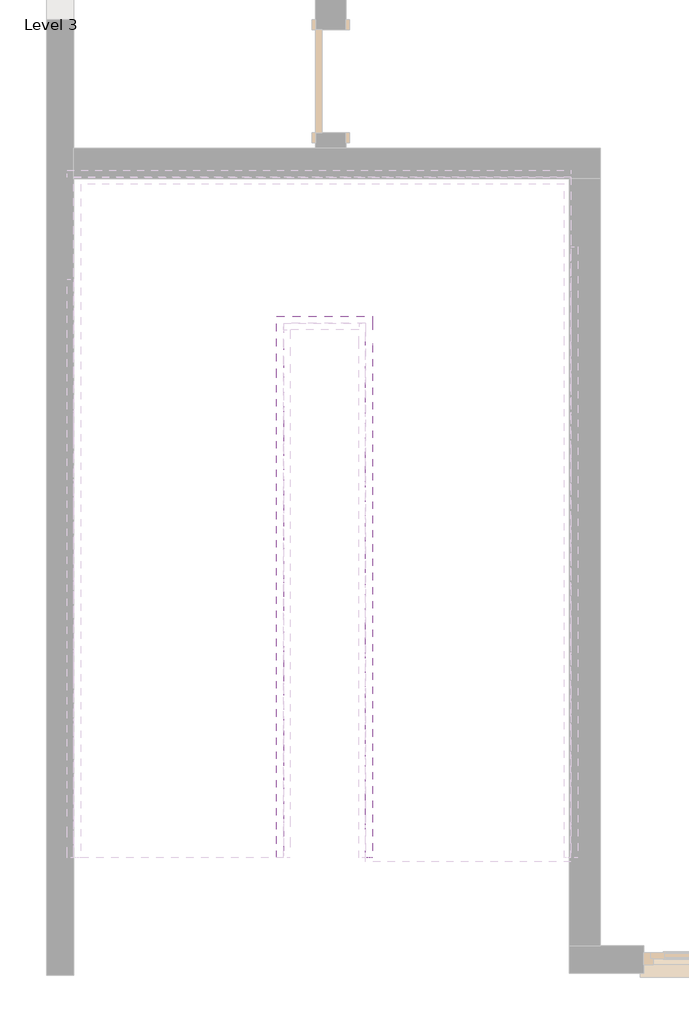
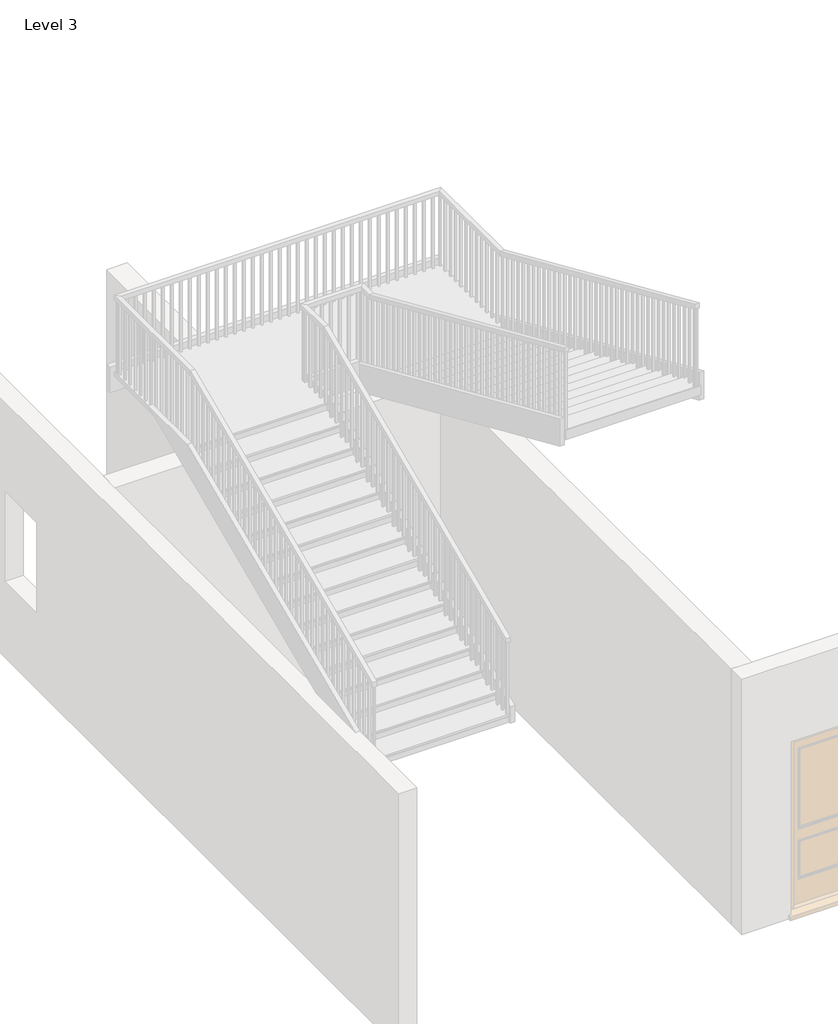
# One storey, part 4 of 6: 1 railing.
"""IFC4 building model written with IfcOpenShell, lengths in millimetres."""

from ifc_helpers import new_model, si_unit, frame, origin, place, context, project, spatial, polyline, outline, extrude, faceted_brep, element, save

model = new_model("IFC4")

# Units and contexts
model_context = context("Model", 3, world=origin())
ifc_project = project(units=[si_unit("LENGTHUNIT", "METRE", prefix="MILLI")], contexts=[model_context])

# Site, building, storey
site = spatial("IfcSite", under=ifc_project)
building = spatial("IfcBuilding", under=site)
storey = spatial("IfcBuildingStorey", under=building, Name="Level 3", Elevation=6096.0)

# Railing
placement = place(None, origin())
element("IfcRailing", 1, ObjectType="Handrail - Rectangular", at=placement, inside=storey, context=model_context, shape_type="SolidModel", body=[
    faceted_brep([(-6050.7290366, -6973.0610642, 9865.36), (-6050.7290366, -6973.0610642, 9809.8599828), (-5999.9290366, -6973.0610642, 9809.8599828), (-5999.9290366, -6973.0610642, 9865.36), (-6050.7290366, -3417.0610642, 11430.0), (-6050.7290366, -3406.3792071, 11379.2), (-5999.9290366, -3406.3792071, 11379.2), (-5999.9290366, -3417.0610642, 11430.0), (-6050.7290366, -2959.8610642, 11430.0), (-6050.7290366, -2959.8610642, 11379.2), (-5999.9290366, -3010.6610642, 11379.2), (-5999.9290366, -3010.6610642, 11430.0), (-5339.5290366, -2959.8610642, 11430.0), (-5339.5290366, -2959.8610642, 11379.2), (-5390.3290366, -3010.6610642, 11379.2), (-5390.3290366, -3010.6610642, 11430.0), (-5339.5290366, -3163.0610642, 11430.0), (-5339.5290366, -3173.7429214, 11379.2), (-5390.3290366, -3173.7429214, 11379.2), (-5390.3290366, -3163.0610642, 11430.0), (-5339.5290366, -6973.0610642, 13106.4), (-5390.3290366, -6973.0610642, 13106.4), (-5390.3290366, -6973.0610642, 13050.8999828), (-5339.5290366, -6973.0610642, 13050.8999828)], [[[0, 1, 2, 3]], [[1, 0, 4, 5]], [[2, 1, 5, 6]], [[3, 2, 6, 7]], [[0, 3, 7, 4]], [[5, 4, 8, 9]], [[6, 5, 9, 10]], [[7, 6, 10, 11]], [[4, 7, 11, 8]], [[9, 8, 12, 13]], [[10, 9, 13, 14]], [[11, 10, 14, 15]], [[8, 11, 15, 12]], [[13, 12, 16, 17]], [[14, 13, 17, 18]], [[15, 14, 18, 19]], [[12, 15, 19, 16]], [[20, 21, 22, 23]], [[17, 16, 20, 23]], [[18, 17, 23, 22]], [[19, 18, 22, 21]], [[16, 19, 21, 20]]]),
    extrude(outline(polyline([(-6957.1860642, 13043.9149828), (-6938.1360642, 13035.5329828), (-6938.1360642, 12080.24), (-6957.1860642, 12080.24), (-6957.1860642, 13043.9149828)])), frame((-5374.4540366, 0.0, 0.0), z_axis=(1.0, 0.0, 0.0), x_axis=(0.0, 1.0, 0.0)), (0.0, 0.0, 1.0), 19.05),
    extrude(outline(polyline([(-6855.5860642, 12999.2109828), (-6836.5360642, 12990.8289828), (-6836.5360642, 12080.24), (-6855.5860642, 12080.24), (-6855.5860642, 12999.2109828)])), frame((-5374.4540366, 0.0, 0.0), z_axis=(1.0, 0.0, 0.0), x_axis=(0.0, 1.0, 0.0)), (0.0, 0.0, 1.0), 19.05),
    extrude(outline(polyline([(-6753.9860642, 12954.5069828), (-6734.9360642, 12946.1249828), (-6734.9360642, 12080.24), (-6753.9860642, 12080.24), (-6753.9860642, 12954.5069828)])), frame((-5374.4540366, 0.0, 0.0), z_axis=(1.0, 0.0, 0.0), x_axis=(0.0, 1.0, 0.0)), (0.0, 0.0, 1.0), 19.05),
    extrude(outline(polyline([(-6652.3860642, 12909.8029828), (-6633.3360642, 12901.4209828), (-6633.3360642, 11968.48), (-6652.3860642, 11968.48), (-6652.3860642, 12909.8029828)])), frame((-5374.4540366, 0.0, 0.0), z_axis=(1.0, 0.0, 0.0), x_axis=(0.0, 1.0, 0.0)), (0.0, 0.0, 1.0), 19.05),
    extrude(outline(polyline([(-6550.7860642, 12865.0989828), (-6531.7360642, 12856.7169828), (-6531.7360642, 11968.48), (-6550.7860642, 11968.48), (-6550.7860642, 12865.0989828)])), frame((-5374.4540366, 0.0, 0.0), z_axis=(1.0, 0.0, 0.0), x_axis=(0.0, 1.0, 0.0)), (0.0, 0.0, 1.0), 19.05),
    extrude(outline(polyline([(-6449.1860642, 12820.3949828), (-6430.1360642, 12812.0129828), (-6430.1360642, 11856.72), (-6449.1860642, 11856.72), (-6449.1860642, 12820.3949828)])), frame((-5374.4540366, 0.0, 0.0), z_axis=(1.0, 0.0, 0.0), x_axis=(0.0, 1.0, 0.0)), (0.0, 0.0, 1.0), 19.05),
    extrude(outline(polyline([(-6347.5860642, 12775.6909828), (-6328.5360642, 12767.3089828), (-6328.5360642, 11856.72), (-6347.5860642, 11856.72), (-6347.5860642, 12775.6909828)])), frame((-5374.4540366, 0.0, 0.0), z_axis=(1.0, 0.0, 0.0), x_axis=(0.0, 1.0, 0.0)), (0.0, 0.0, 1.0), 19.05),
    extrude(outline(polyline([(-6245.9860642, 12730.9869828), (-6226.9360642, 12722.6049828), (-6226.9360642, 11856.72), (-6245.9860642, 11856.72), (-6245.9860642, 12730.9869828)])), frame((-5374.4540366, 0.0, 0.0), z_axis=(1.0, 0.0, 0.0), x_axis=(0.0, 1.0, 0.0)), (0.0, 0.0, 1.0), 19.05),
    extrude(outline(polyline([(-6144.3860642, 12686.2829828), (-6125.3360642, 12677.9009828), (-6125.3360642, 11744.96), (-6144.3860642, 11744.96), (-6144.3860642, 12686.2829828)])), frame((-5374.4540366, 0.0, 0.0), z_axis=(1.0, 0.0, 0.0), x_axis=(0.0, 1.0, 0.0)), (0.0, 0.0, 1.0), 19.05),
    extrude(outline(polyline([(-6042.7860642, 12641.5789828), (-6023.7360642, 12633.1969828), (-6023.7360642, 11744.96), (-6042.7860642, 11744.96), (-6042.7860642, 12641.5789828)])), frame((-5374.4540366, 0.0, 0.0), z_axis=(1.0, 0.0, 0.0), x_axis=(0.0, 1.0, 0.0)), (0.0, 0.0, 1.0), 19.05),
    extrude(outline(polyline([(-5941.1860642, 12596.8749828), (-5922.1360642, 12588.4929828), (-5922.1360642, 11633.2), (-5941.1860642, 11633.2), (-5941.1860642, 12596.8749828)])), frame((-5374.4540366, 0.0, 0.0), z_axis=(1.0, 0.0, 0.0), x_axis=(0.0, 1.0, 0.0)), (0.0, 0.0, 1.0), 19.05),
    extrude(outline(polyline([(-5839.5860642, 12552.1709828), (-5820.5360642, 12543.7889828), (-5820.5360642, 11633.2), (-5839.5860642, 11633.2), (-5839.5860642, 12552.1709828)])), frame((-5374.4540366, 0.0, 0.0), z_axis=(1.0, 0.0, 0.0), x_axis=(0.0, 1.0, 0.0)), (0.0, 0.0, 1.0), 19.05),
    extrude(outline(polyline([(-5737.9860642, 12507.4669828), (-5718.9360642, 12499.0849828), (-5718.9360642, 11633.2), (-5737.9860642, 11633.2), (-5737.9860642, 12507.4669828)])), frame((-5374.4540366, 0.0, 0.0), z_axis=(1.0, 0.0, 0.0), x_axis=(0.0, 1.0, 0.0)), (0.0, 0.0, 1.0), 19.05),
    extrude(outline(polyline([(-5636.3860642, 12462.7629828), (-5617.3360642, 12454.3809828), (-5617.3360642, 11521.44), (-5636.3860642, 11521.44), (-5636.3860642, 12462.7629828)])), frame((-5374.4540366, 0.0, 0.0), z_axis=(1.0, 0.0, 0.0), x_axis=(0.0, 1.0, 0.0)), (0.0, 0.0, 1.0), 19.05),
    extrude(outline(polyline([(-5534.7860642, 12418.0589828), (-5515.7360642, 12409.6769828), (-5515.7360642, 11521.44), (-5534.7860642, 11521.44), (-5534.7860642, 12418.0589828)])), frame((-5374.4540366, 0.0, 0.0), z_axis=(1.0, 0.0, 0.0), x_axis=(0.0, 1.0, 0.0)), (0.0, 0.0, 1.0), 19.05),
    extrude(outline(polyline([(-5433.1860642, 12373.3549828), (-5414.1360642, 12364.9729828), (-5414.1360642, 11409.68), (-5433.1860642, 11409.68), (-5433.1860642, 12373.3549828)])), frame((-5374.4540366, 0.0, 0.0), z_axis=(1.0, 0.0, 0.0), x_axis=(0.0, 1.0, 0.0)), (0.0, 0.0, 1.0), 19.05),
    extrude(outline(polyline([(-5331.5860642, 12328.6509828), (-5312.5360642, 12320.2689828), (-5312.5360642, 11409.68), (-5331.5860642, 11409.68), (-5331.5860642, 12328.6509828)])), frame((-5374.4540366, 0.0, 0.0), z_axis=(1.0, 0.0, 0.0), x_axis=(0.0, 1.0, 0.0)), (0.0, 0.0, 1.0), 19.05),
    extrude(outline(polyline([(-5229.9860642, 12283.9469828), (-5210.9360642, 12275.5649828), (-5210.9360642, 11409.68), (-5229.9860642, 11409.68), (-5229.9860642, 12283.9469828)])), frame((-5374.4540366, 0.0, 0.0), z_axis=(1.0, 0.0, 0.0), x_axis=(0.0, 1.0, 0.0)), (0.0, 0.0, 1.0), 19.05),
    extrude(outline(polyline([(-5128.3860642, 12239.2429828), (-5109.3360642, 12230.8609828), (-5109.3360642, 11297.92), (-5128.3860642, 11297.92), (-5128.3860642, 12239.2429828)])), frame((-5374.4540366, 0.0, 0.0), z_axis=(1.0, 0.0, 0.0), x_axis=(0.0, 1.0, 0.0)), (0.0, 0.0, 1.0), 19.05),
    extrude(outline(polyline([(-5026.7860642, 12194.5389828), (-5007.7360642, 12186.1569828), (-5007.7360642, 11297.92), (-5026.7860642, 11297.92), (-5026.7860642, 12194.5389828)])), frame((-5374.4540366, 0.0, 0.0), z_axis=(1.0, 0.0, 0.0), x_axis=(0.0, 1.0, 0.0)), (0.0, 0.0, 1.0), 19.05),
    extrude(outline(polyline([(-4925.1860642, 12149.8349828), (-4906.1360642, 12141.4529828), (-4906.1360642, 11186.16), (-4925.1860642, 11186.16), (-4925.1860642, 12149.8349828)])), frame((-5374.4540366, 0.0, 0.0), z_axis=(1.0, 0.0, 0.0), x_axis=(0.0, 1.0, 0.0)), (0.0, 0.0, 1.0), 19.05),
    extrude(outline(polyline([(-4823.5860642, 12105.1309828), (-4804.5360642, 12096.7489828), (-4804.5360642, 11186.16), (-4823.5860642, 11186.16), (-4823.5860642, 12105.1309828)])), frame((-5374.4540366, 0.0, 0.0), z_axis=(1.0, 0.0, 0.0), x_axis=(0.0, 1.0, 0.0)), (0.0, 0.0, 1.0), 19.05),
    extrude(outline(polyline([(-4721.9860642, 12060.4269828), (-4702.9360642, 12052.0449828), (-4702.9360642, 11186.16), (-4721.9860642, 11186.16), (-4721.9860642, 12060.4269828)])), frame((-5374.4540366, 0.0, 0.0), z_axis=(1.0, 0.0, 0.0), x_axis=(0.0, 1.0, 0.0)), (0.0, 0.0, 1.0), 19.05),
    extrude(outline(polyline([(-4620.3860642, 12015.7229828), (-4601.3360642, 12007.3409828), (-4601.3360642, 11074.4), (-4620.3860642, 11074.4), (-4620.3860642, 12015.7229828)])), frame((-5374.4540366, 0.0, 0.0), z_axis=(1.0, 0.0, 0.0), x_axis=(0.0, 1.0, 0.0)), (0.0, 0.0, 1.0), 19.05),
    extrude(outline(polyline([(-4518.7860642, 11971.0189828), (-4499.7360642, 11962.6369828), (-4499.7360642, 11074.4), (-4518.7860642, 11074.4), (-4518.7860642, 11971.0189828)])), frame((-5374.4540366, 0.0, 0.0), z_axis=(1.0, 0.0, 0.0), x_axis=(0.0, 1.0, 0.0)), (0.0, 0.0, 1.0), 19.05),
    extrude(outline(polyline([(-4417.1860642, 11926.3149828), (-4398.1360642, 11917.9329828), (-4398.1360642, 10962.64), (-4417.1860642, 10962.64), (-4417.1860642, 11926.3149828)])), frame((-5374.4540366, 0.0, 0.0), z_axis=(1.0, 0.0, 0.0), x_axis=(0.0, 1.0, 0.0)), (0.0, 0.0, 1.0), 19.05),
    extrude(outline(polyline([(-4315.5860642, 11881.6109828), (-4296.5360642, 11873.2289828), (-4296.5360642, 10962.64), (-4315.5860642, 10962.64), (-4315.5860642, 11881.6109828)])), frame((-5374.4540366, 0.0, 0.0), z_axis=(1.0, 0.0, 0.0), x_axis=(0.0, 1.0, 0.0)), (0.0, 0.0, 1.0), 19.05),
    extrude(outline(polyline([(-4213.9860642, 11836.9069828), (-4194.9360642, 11828.5249828), (-4194.9360642, 10962.64), (-4213.9860642, 10962.64), (-4213.9860642, 11836.9069828)])), frame((-5374.4540366, 0.0, 0.0), z_axis=(1.0, 0.0, 0.0), x_axis=(0.0, 1.0, 0.0)), (0.0, 0.0, 1.0), 19.05),
    extrude(outline(polyline([(-4112.3860642, 11792.2029828), (-4093.3360642, 11783.8209828), (-4093.3360642, 10850.88), (-4112.3860642, 10850.88), (-4112.3860642, 11792.2029828)])), frame((-5374.4540366, 0.0, 0.0), z_axis=(1.0, 0.0, 0.0), x_axis=(0.0, 1.0, 0.0)), (0.0, 0.0, 1.0), 19.05),
    extrude(outline(polyline([(-4010.7860642, 11747.4989828), (-3991.7360642, 11739.1169828), (-3991.7360642, 10850.88), (-4010.7860642, 10850.88), (-4010.7860642, 11747.4989828)])), frame((-5374.4540366, 0.0, 0.0), z_axis=(1.0, 0.0, 0.0), x_axis=(0.0, 1.0, 0.0)), (0.0, 0.0, 1.0), 19.05),
    extrude(outline(polyline([(-3909.1860642, 11702.7949828), (-3890.1360642, 11694.4129828), (-3890.1360642, 10739.12), (-3909.1860642, 10739.12), (-3909.1860642, 11702.7949828)])), frame((-5374.4540366, 0.0, 0.0), z_axis=(1.0, 0.0, 0.0), x_axis=(0.0, 1.0, 0.0)), (0.0, 0.0, 1.0), 19.05),
    extrude(outline(polyline([(-3807.5860642, 11658.0909828), (-3788.5360642, 11649.7089828), (-3788.5360642, 10739.12), (-3807.5860642, 10739.12), (-3807.5860642, 11658.0909828)])), frame((-5374.4540366, 0.0, 0.0), z_axis=(1.0, 0.0, 0.0), x_axis=(0.0, 1.0, 0.0)), (0.0, 0.0, 1.0), 19.05),
    extrude(outline(polyline([(-3705.9860642, 11613.3869828), (-3686.9360642, 11605.0049828), (-3686.9360642, 10739.12), (-3705.9860642, 10739.12), (-3705.9860642, 11613.3869828)])), frame((-5374.4540366, 0.0, 0.0), z_axis=(1.0, 0.0, 0.0), x_axis=(0.0, 1.0, 0.0)), (0.0, 0.0, 1.0), 19.05),
    extrude(outline(polyline([(-3604.3860642, 11568.6829828), (-3585.3360642, 11560.3009828), (-3585.3360642, 10627.36), (-3604.3860642, 10627.36), (-3604.3860642, 11568.6829828)])), frame((-5374.4540366, 0.0, 0.0), z_axis=(1.0, 0.0, 0.0), x_axis=(0.0, 1.0, 0.0)), (0.0, 0.0, 1.0), 19.05),
    extrude(outline(polyline([(-3502.7860642, 11523.9789828), (-3483.7360642, 11515.5969828), (-3483.7360642, 10627.36), (-3502.7860642, 10627.36), (-3502.7860642, 11523.9789828)])), frame((-5374.4540366, 0.0, 0.0), z_axis=(1.0, 0.0, 0.0), x_axis=(0.0, 1.0, 0.0)), (0.0, 0.0, 1.0), 19.05),
    extrude(outline(polyline([(-3401.1860642, 11479.2749828), (-3382.1360642, 11470.8929828), (-3382.1360642, 10515.6), (-3401.1860642, 10515.6), (-3401.1860642, 11479.2749828)])), frame((-5374.4540366, 0.0, 0.0), z_axis=(1.0, 0.0, 0.0), x_axis=(0.0, 1.0, 0.0)), (0.0, 0.0, 1.0), 19.05),
    extrude(outline(polyline([(-3299.5860642, 11434.5709828), (-3280.5360642, 11426.1889828), (-3280.5360642, 10515.6), (-3299.5860642, 10515.6), (-3299.5860642, 11434.5709828)])), frame((-5374.4540366, 0.0, 0.0), z_axis=(1.0, 0.0, 0.0), x_axis=(0.0, 1.0, 0.0)), (0.0, 0.0, 1.0), 19.05),
    extrude(outline(polyline([(-3197.9860642, 11389.8669828), (-3178.9360642, 11381.4849828), (-3178.9360642, 10515.6), (-3197.9860642, 10515.6), (-3197.9860642, 11389.8669828)])), frame((-5374.4540366, 0.0, 0.0), z_axis=(1.0, 0.0, 0.0), x_axis=(0.0, 1.0, 0.0)), (0.0, 0.0, 1.0), 19.05),
    extrude(outline(polyline([(-5374.4540366, -3077.3360642), (-5355.4040366, -3077.3360642), (-5355.4040366, -3096.3860642), (-5374.4540366, -3096.3860642), (-5374.4540366, -3077.3360642)])), frame((0.0, 0.0, 10515.6), z_axis=(0.0, 0.0, 1.0), x_axis=(1.0, 0.0, 0.0)), (0.0, 0.0, 1.0), 863.6),
    extrude(outline(polyline([(-5425.2540366, -2994.7860642), (-5425.2540366, -2975.7360642), (-5406.2040366, -2975.7360642), (-5406.2040366, -2994.7860642), (-5425.2540366, -2994.7860642)])), frame((0.0, 0.0, 10515.6), z_axis=(0.0, 0.0, 1.0), x_axis=(1.0, 0.0, 0.0)), (0.0, 0.0, 1.0), 863.6),
    extrude(outline(polyline([(-5526.8540366, -2994.7860642), (-5526.8540366, -2975.7360642), (-5507.8040366, -2975.7360642), (-5507.8040366, -2994.7860642), (-5526.8540366, -2994.7860642)])), frame((0.0, 0.0, 10515.6), z_axis=(0.0, 0.0, 1.0), x_axis=(1.0, 0.0, 0.0)), (0.0, 0.0, 1.0), 863.6),
    extrude(outline(polyline([(-5628.4540366, -2994.7860642), (-5628.4540366, -2975.7360642), (-5609.4040366, -2975.7360642), (-5609.4040366, -2994.7860642), (-5628.4540366, -2994.7860642)])), frame((0.0, 0.0, 10515.6), z_axis=(0.0, 0.0, 1.0), x_axis=(1.0, 0.0, 0.0)), (0.0, 0.0, 1.0), 863.6),
    extrude(outline(polyline([(-5730.0540366, -2994.7860642), (-5730.0540366, -2975.7360642), (-5711.0040366, -2975.7360642), (-5711.0040366, -2994.7860642), (-5730.0540366, -2994.7860642)])), frame((0.0, 0.0, 10515.6), z_axis=(0.0, 0.0, 1.0), x_axis=(1.0, 0.0, 0.0)), (0.0, 0.0, 1.0), 863.6),
    extrude(outline(polyline([(-5831.6540366, -2994.7860642), (-5831.6540366, -2975.7360642), (-5812.6040366, -2975.7360642), (-5812.6040366, -2994.7860642), (-5831.6540366, -2994.7860642)])), frame((0.0, 0.0, 10515.6), z_axis=(0.0, 0.0, 1.0), x_axis=(1.0, 0.0, 0.0)), (0.0, 0.0, 1.0), 863.6),
    extrude(outline(polyline([(-5933.2540366, -2994.7860642), (-5933.2540366, -2975.7360642), (-5914.2040366, -2975.7360642), (-5914.2040366, -2994.7860642), (-5933.2540366, -2994.7860642)])), frame((0.0, 0.0, 10515.6), z_axis=(0.0, 0.0, 1.0), x_axis=(1.0, 0.0, 0.0)), (0.0, 0.0, 1.0), 863.6),
    extrude(outline(polyline([(-6015.8040366, -3020.1860642), (-6034.8540366, -3020.1860642), (-6034.8540366, -3001.1360642), (-6015.8040366, -3001.1360642), (-6015.8040366, -3020.1860642)])), frame((0.0, 0.0, 10515.6), z_axis=(0.0, 0.0, 1.0), x_axis=(1.0, 0.0, 0.0)), (0.0, 0.0, 1.0), 863.6),
    extrude(outline(polyline([(-6015.8040366, -3121.7860642), (-6034.8540366, -3121.7860642), (-6034.8540366, -3102.7360642), (-6015.8040366, -3102.7360642), (-6015.8040366, -3121.7860642)])), frame((0.0, 0.0, 10515.6), z_axis=(0.0, 0.0, 1.0), x_axis=(1.0, 0.0, 0.0)), (0.0, 0.0, 1.0), 863.6),
    extrude(outline(polyline([(-6015.8040366, -3223.3860642), (-6034.8540366, -3223.3860642), (-6034.8540366, -3204.3360642), (-6015.8040366, -3204.3360642), (-6015.8040366, -3223.3860642)])), frame((0.0, 0.0, 10515.6), z_axis=(0.0, 0.0, 1.0), x_axis=(1.0, 0.0, 0.0)), (0.0, 0.0, 1.0), 863.6),
    extrude(outline(polyline([(-6015.8040366, -3324.9860642), (-6034.8540366, -3324.9860642), (-6034.8540366, -3305.9360642), (-6015.8040366, -3305.9360642), (-6015.8040366, -3324.9860642)])), frame((0.0, 0.0, 10515.6), z_axis=(0.0, 0.0, 1.0), x_axis=(1.0, 0.0, 0.0)), (0.0, 0.0, 1.0), 863.6),
    extrude(outline(polyline([(-3426.5860642, 11370.3089828), (-3407.5360642, 11378.6909828), (-3407.5360642, 10515.6), (-3426.5860642, 10515.6), (-3426.5860642, 11370.3089828)])), frame((-6034.8540366, 0.0, 0.0), z_axis=(1.0, 0.0, 0.0), x_axis=(0.0, 1.0, 0.0)), (0.0, 0.0, 1.0), 19.05),
    extrude(outline(polyline([(-3528.1860642, 11325.6049828), (-3509.1360642, 11333.9869828), (-3509.1360642, 10403.84), (-3528.1860642, 10403.84), (-3528.1860642, 11325.6049828)])), frame((-6034.8540366, 0.0, 0.0), z_axis=(1.0, 0.0, 0.0), x_axis=(0.0, 1.0, 0.0)), (0.0, 0.0, 1.0), 19.05),
    extrude(outline(polyline([(-3629.7860642, 11280.9009828), (-3610.7360642, 11289.2829828), (-3610.7360642, 10403.84), (-3629.7860642, 10403.84), (-3629.7860642, 11280.9009828)])), frame((-6034.8540366, 0.0, 0.0), z_axis=(1.0, 0.0, 0.0), x_axis=(0.0, 1.0, 0.0)), (0.0, 0.0, 1.0), 19.05),
    extrude(outline(polyline([(-3731.3860642, 11236.1969828), (-3712.3360642, 11244.5789828), (-3712.3360642, 10292.08), (-3731.3860642, 10292.08), (-3731.3860642, 11236.1969828)])), frame((-6034.8540366, 0.0, 0.0), z_axis=(1.0, 0.0, 0.0), x_axis=(0.0, 1.0, 0.0)), (0.0, 0.0, 1.0), 19.05),
    extrude(outline(polyline([(-3832.9860642, 11191.4929828), (-3813.9360642, 11199.8749828), (-3813.9360642, 10292.08), (-3832.9860642, 10292.08), (-3832.9860642, 11191.4929828)])), frame((-6034.8540366, 0.0, 0.0), z_axis=(1.0, 0.0, 0.0), x_axis=(0.0, 1.0, 0.0)), (0.0, 0.0, 1.0), 19.05),
    extrude(outline(polyline([(-3934.5860642, 11146.7889828), (-3915.5360642, 11155.1709828), (-3915.5360642, 10292.08), (-3934.5860642, 10292.08), (-3934.5860642, 11146.7889828)])), frame((-6034.8540366, 0.0, 0.0), z_axis=(1.0, 0.0, 0.0), x_axis=(0.0, 1.0, 0.0)), (0.0, 0.0, 1.0), 19.05),
    extrude(outline(polyline([(-4036.1860642, 11102.0849828), (-4017.1360642, 11110.4669828), (-4017.1360642, 10180.32), (-4036.1860642, 10180.32), (-4036.1860642, 11102.0849828)])), frame((-6034.8540366, 0.0, 0.0), z_axis=(1.0, 0.0, 0.0), x_axis=(0.0, 1.0, 0.0)), (0.0, 0.0, 1.0), 19.05),
    extrude(outline(polyline([(-4137.7860642, 11057.3809828), (-4118.7360642, 11065.7629828), (-4118.7360642, 10180.32), (-4137.7860642, 10180.32), (-4137.7860642, 11057.3809828)])), frame((-6034.8540366, 0.0, 0.0), z_axis=(1.0, 0.0, 0.0), x_axis=(0.0, 1.0, 0.0)), (0.0, 0.0, 1.0), 19.05),
    extrude(outline(polyline([(-4239.3860642, 11012.6769828), (-4220.3360642, 11021.0589828), (-4220.3360642, 10068.56), (-4239.3860642, 10068.56), (-4239.3860642, 11012.6769828)])), frame((-6034.8540366, 0.0, 0.0), z_axis=(1.0, 0.0, 0.0), x_axis=(0.0, 1.0, 0.0)), (0.0, 0.0, 1.0), 19.05),
    extrude(outline(polyline([(-4340.9860642, 10967.9729828), (-4321.9360642, 10976.3549828), (-4321.9360642, 10068.56), (-4340.9860642, 10068.56), (-4340.9860642, 10967.9729828)])), frame((-6034.8540366, 0.0, 0.0), z_axis=(1.0, 0.0, 0.0), x_axis=(0.0, 1.0, 0.0)), (0.0, 0.0, 1.0), 19.05),
    extrude(outline(polyline([(-4442.5860642, 10923.2689828), (-4423.5360642, 10931.6509828), (-4423.5360642, 10068.56), (-4442.5860642, 10068.56), (-4442.5860642, 10923.2689828)])), frame((-6034.8540366, 0.0, 0.0), z_axis=(1.0, 0.0, 0.0), x_axis=(0.0, 1.0, 0.0)), (0.0, 0.0, 1.0), 19.05),
    extrude(outline(polyline([(-4544.1860642, 10878.5649828), (-4525.1360642, 10886.9469828), (-4525.1360642, 9956.8), (-4544.1860642, 9956.8), (-4544.1860642, 10878.5649828)])), frame((-6034.8540366, 0.0, 0.0), z_axis=(1.0, 0.0, 0.0), x_axis=(0.0, 1.0, 0.0)), (0.0, 0.0, 1.0), 19.05),
    extrude(outline(polyline([(-4645.7860642, 10833.8609828), (-4626.7360642, 10842.2429828), (-4626.7360642, 9956.8), (-4645.7860642, 9956.8), (-4645.7860642, 10833.8609828)])), frame((-6034.8540366, 0.0, 0.0), z_axis=(1.0, 0.0, 0.0), x_axis=(0.0, 1.0, 0.0)), (0.0, 0.0, 1.0), 19.05),
    extrude(outline(polyline([(-4747.3860642, 10789.1569828), (-4728.3360642, 10797.5389828), (-4728.3360642, 9845.04), (-4747.3860642, 9845.04), (-4747.3860642, 10789.1569828)])), frame((-6034.8540366, 0.0, 0.0), z_axis=(1.0, 0.0, 0.0), x_axis=(0.0, 1.0, 0.0)), (0.0, 0.0, 1.0), 19.05),
    extrude(outline(polyline([(-4848.9860642, 10744.4529828), (-4829.9360642, 10752.8349828), (-4829.9360642, 9845.04), (-4848.9860642, 9845.04), (-4848.9860642, 10744.4529828)])), frame((-6034.8540366, 0.0, 0.0), z_axis=(1.0, 0.0, 0.0), x_axis=(0.0, 1.0, 0.0)), (0.0, 0.0, 1.0), 19.05),
    extrude(outline(polyline([(-4950.5860642, 10699.7489828), (-4931.5360642, 10708.1309828), (-4931.5360642, 9845.04), (-4950.5860642, 9845.04), (-4950.5860642, 10699.7489828)])), frame((-6034.8540366, 0.0, 0.0), z_axis=(1.0, 0.0, 0.0), x_axis=(0.0, 1.0, 0.0)), (0.0, 0.0, 1.0), 19.05),
    extrude(outline(polyline([(-5052.1860642, 10655.0449828), (-5033.1360642, 10663.4269828), (-5033.1360642, 9733.28), (-5052.1860642, 9733.28), (-5052.1860642, 10655.0449828)])), frame((-6034.8540366, 0.0, 0.0), z_axis=(1.0, 0.0, 0.0), x_axis=(0.0, 1.0, 0.0)), (0.0, 0.0, 1.0), 19.05),
    extrude(outline(polyline([(-5153.7860642, 10610.3409828), (-5134.7360642, 10618.7229828), (-5134.7360642, 9733.28), (-5153.7860642, 9733.28), (-5153.7860642, 10610.3409828)])), frame((-6034.8540366, 0.0, 0.0), z_axis=(1.0, 0.0, 0.0), x_axis=(0.0, 1.0, 0.0)), (0.0, 0.0, 1.0), 19.05),
    extrude(outline(polyline([(-5255.3860642, 10565.6369828), (-5236.3360642, 10574.0189828), (-5236.3360642, 9621.52), (-5255.3860642, 9621.52), (-5255.3860642, 10565.6369828)])), frame((-6034.8540366, 0.0, 0.0), z_axis=(1.0, 0.0, 0.0), x_axis=(0.0, 1.0, 0.0)), (0.0, 0.0, 1.0), 19.05),
    extrude(outline(polyline([(-5356.9860642, 10520.9329828), (-5337.9360642, 10529.3149828), (-5337.9360642, 9621.52), (-5356.9860642, 9621.52), (-5356.9860642, 10520.9329828)])), frame((-6034.8540366, 0.0, 0.0), z_axis=(1.0, 0.0, 0.0), x_axis=(0.0, 1.0, 0.0)), (0.0, 0.0, 1.0), 19.05),
    extrude(outline(polyline([(-5458.5860642, 10476.2289828), (-5439.5360642, 10484.6109828), (-5439.5360642, 9621.52), (-5458.5860642, 9621.52), (-5458.5860642, 10476.2289828)])), frame((-6034.8540366, 0.0, 0.0), z_axis=(1.0, 0.0, 0.0), x_axis=(0.0, 1.0, 0.0)), (0.0, 0.0, 1.0), 19.05),
    extrude(outline(polyline([(-5560.1860642, 10431.5249828), (-5541.1360642, 10439.9069828), (-5541.1360642, 9509.76), (-5560.1860642, 9509.76), (-5560.1860642, 10431.5249828)])), frame((-6034.8540366, 0.0, 0.0), z_axis=(1.0, 0.0, 0.0), x_axis=(0.0, 1.0, 0.0)), (0.0, 0.0, 1.0), 19.05),
    extrude(outline(polyline([(-5661.7860642, 10386.8209828), (-5642.7360642, 10395.2029828), (-5642.7360642, 9509.76), (-5661.7860642, 9509.76), (-5661.7860642, 10386.8209828)])), frame((-6034.8540366, 0.0, 0.0), z_axis=(1.0, 0.0, 0.0), x_axis=(0.0, 1.0, 0.0)), (0.0, 0.0, 1.0), 19.05),
    extrude(outline(polyline([(-5763.3860642, 10342.1169828), (-5744.3360642, 10350.4989828), (-5744.3360642, 9398.0), (-5763.3860642, 9398.0), (-5763.3860642, 10342.1169828)])), frame((-6034.8540366, 0.0, 0.0), z_axis=(1.0, 0.0, 0.0), x_axis=(0.0, 1.0, 0.0)), (0.0, 0.0, 1.0), 19.05),
    extrude(outline(polyline([(-5864.9860642, 10297.4129828), (-5845.9360642, 10305.7949828), (-5845.9360642, 9398.0), (-5864.9860642, 9398.0), (-5864.9860642, 10297.4129828)])), frame((-6034.8540366, 0.0, 0.0), z_axis=(1.0, 0.0, 0.0), x_axis=(0.0, 1.0, 0.0)), (0.0, 0.0, 1.0), 19.05),
    extrude(outline(polyline([(-5966.5860642, 10252.7089828), (-5947.5360642, 10261.0909828), (-5947.5360642, 9398.0), (-5966.5860642, 9398.0), (-5966.5860642, 10252.7089828)])), frame((-6034.8540366, 0.0, 0.0), z_axis=(1.0, 0.0, 0.0), x_axis=(0.0, 1.0, 0.0)), (0.0, 0.0, 1.0), 19.05),
    extrude(outline(polyline([(-6068.1860642, 10208.0049828), (-6049.1360642, 10216.3869828), (-6049.1360642, 9286.24), (-6068.1860642, 9286.24), (-6068.1860642, 10208.0049828)])), frame((-6034.8540366, 0.0, 0.0), z_axis=(1.0, 0.0, 0.0), x_axis=(0.0, 1.0, 0.0)), (0.0, 0.0, 1.0), 19.05),
    extrude(outline(polyline([(-6169.7860642, 10163.3009828), (-6150.7360642, 10171.6829828), (-6150.7360642, 9286.24), (-6169.7860642, 9286.24), (-6169.7860642, 10163.3009828)])), frame((-6034.8540366, 0.0, 0.0), z_axis=(1.0, 0.0, 0.0), x_axis=(0.0, 1.0, 0.0)), (0.0, 0.0, 1.0), 19.05),
    extrude(outline(polyline([(-6271.3860642, 10118.5969828), (-6252.3360642, 10126.9789828), (-6252.3360642, 9174.48), (-6271.3860642, 9174.48), (-6271.3860642, 10118.5969828)])), frame((-6034.8540366, 0.0, 0.0), z_axis=(1.0, 0.0, 0.0), x_axis=(0.0, 1.0, 0.0)), (0.0, 0.0, 1.0), 19.05),
    extrude(outline(polyline([(-6372.9860642, 10073.8929828), (-6353.9360642, 10082.2749828), (-6353.9360642, 9174.48), (-6372.9860642, 9174.48), (-6372.9860642, 10073.8929828)])), frame((-6034.8540366, 0.0, 0.0), z_axis=(1.0, 0.0, 0.0), x_axis=(0.0, 1.0, 0.0)), (0.0, 0.0, 1.0), 19.05),
    extrude(outline(polyline([(-6474.5860642, 10029.1889828), (-6455.5360642, 10037.5709828), (-6455.5360642, 9174.48), (-6474.5860642, 9174.48), (-6474.5860642, 10029.1889828)])), frame((-6034.8540366, 0.0, 0.0), z_axis=(1.0, 0.0, 0.0), x_axis=(0.0, 1.0, 0.0)), (0.0, 0.0, 1.0), 19.05),
    extrude(outline(polyline([(-6576.1860642, 9984.4849828), (-6557.1360642, 9992.8669828), (-6557.1360642, 9062.72), (-6576.1860642, 9062.72), (-6576.1860642, 9984.4849828)])), frame((-6034.8540366, 0.0, 0.0), z_axis=(1.0, 0.0, 0.0), x_axis=(0.0, 1.0, 0.0)), (0.0, 0.0, 1.0), 19.05),
    extrude(outline(polyline([(-6677.7860642, 9939.7809828), (-6658.7360642, 9948.1629828), (-6658.7360642, 9062.72), (-6677.7860642, 9062.72), (-6677.7860642, 9939.7809828)])), frame((-6034.8540366, 0.0, 0.0), z_axis=(1.0, 0.0, 0.0), x_axis=(0.0, 1.0, 0.0)), (0.0, 0.0, 1.0), 19.05),
    extrude(outline(polyline([(-6779.3860642, 9895.0769828), (-6760.3360642, 9903.4589828), (-6760.3360642, 8950.96), (-6779.3860642, 8950.96), (-6779.3860642, 9895.0769828)])), frame((-6034.8540366, 0.0, 0.0), z_axis=(1.0, 0.0, 0.0), x_axis=(0.0, 1.0, 0.0)), (0.0, 0.0, 1.0), 19.05),
    extrude(outline(polyline([(-6880.9860642, 9850.3729828), (-6861.9360642, 9858.7549828), (-6861.9360642, 8950.96), (-6880.9860642, 8950.96), (-6880.9860642, 9850.3729828)])), frame((-6034.8540366, 0.0, 0.0), z_axis=(1.0, 0.0, 0.0), x_axis=(0.0, 1.0, 0.0)), (0.0, 0.0, 1.0), 19.05),
    extrude(outline(polyline([(-5374.4540366, -2994.7860642), (-5374.4540366, -2975.7360642), (-5355.4040366, -2975.7360642), (-5355.4040366, -2994.7860642), (-5374.4540366, -2994.7860642)])), frame((0.0, 0.0, 10515.6), z_axis=(0.0, 0.0, 1.0), x_axis=(1.0, 0.0, 0.0)), (0.0, 0.0, 1.0), 863.6),
    extrude(outline(polyline([(-6015.8040366, -2994.7860642), (-6034.8540366, -2994.7860642), (-6034.8540366, -2975.7360642), (-6015.8040366, -2975.7360642), (-6015.8040366, -2994.7860642)])), frame((0.0, 0.0, 10515.6), z_axis=(0.0, 0.0, 1.0), x_axis=(1.0, 0.0, 0.0)), (0.0, 0.0, 1.0), 863.6),
    extrude(outline(polyline([(-6973.0610642, 13050.8999828), (-6954.0110642, 13042.5179828), (-6954.0110642, 12080.24), (-6973.0610642, 12080.24), (-6973.0610642, 13050.8999828)])), frame((-5374.4540366, 0.0, 0.0), z_axis=(1.0, 0.0, 0.0), x_axis=(0.0, 1.0, 0.0)), (0.0, 0.0, 1.0), 19.05),
    extrude(outline(polyline([(-6973.0610642, 9809.8599828), (-6954.0110642, 9818.2419828), (-6954.0110642, 8950.96), (-6973.0610642, 8950.96), (-6973.0610642, 9809.8599828)])), frame((-6034.8540366, 0.0, 0.0), z_axis=(1.0, 0.0, 0.0), x_axis=(0.0, 1.0, 0.0)), (0.0, 0.0, 1.0), 19.05),
])

save(model, "model.ifc")

# Revit data of these elements
# Type "Handrail - Rectangular"
#   Assembly Code = "C2010400"
#   built-in parameter 1008612 = 0.0416667 (stored number, unit not read)
#   built-in parameter 1008611 = 0.0416667 (stored number, unit not read)
#   built-in parameter 1008609 = 0.333333 (stored number, unit not read)
#   built-in parameter 1008604 = 0.166667 (stored number, unit not read)
#   built-in parameter 1008603 = 0.166667 (stored number, unit not read)
#   Railing Height = 3' - 0"
#   built-in parameter 1008630 = 2
#   built-in parameter 1008610 = 2
#   built-in parameter 1008618 = Baluster - Square : 3/4"
# Element 1 (IfcRailing, "Handrail - Rectangular")
#   Phase Created = New Construction
